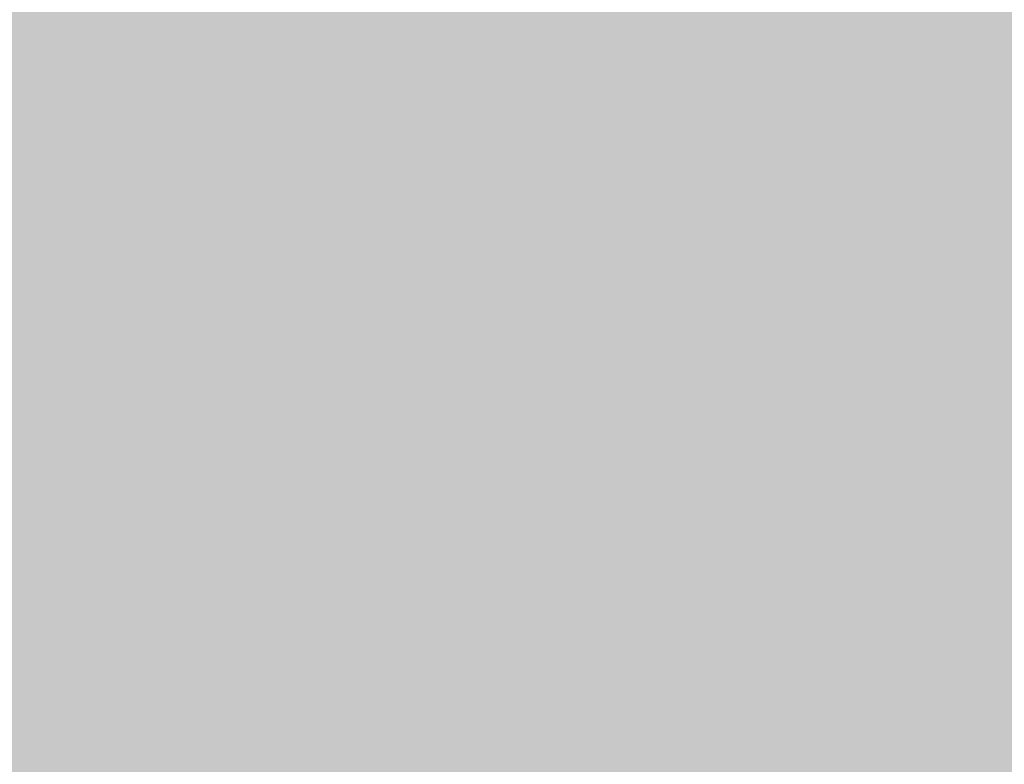
# Model space of a CAD drawing. Units: millimetres. Extents: x 0 to 2267, y 0 to 1823.
# Tile 45 of 256: x 1593.7801 to 1594.2193, y 1226.3857 to 1226.718. Entities that reach past the tile are written whole.
import ezdxf

# ---------------------------------------------------------------- set-up
doc = ezdxf.new("R2010")
doc.units = ezdxf.units.MM
doc.header["$MEASUREMENT"] = 0
doc.layers.add('M-HATC', color=252, linetype='Continuous', lineweight=18)

msp = doc.modelspace()

# ---------------------------------------------------------------- hatches: boundary and pattern name
at = {"layer": 'M-HATC'}
h = msp.add_hatch(color=256, dxfattribs=at)
h.dxf.hatch_style = 1
h.paths.add_polyline_path([(2055.77105, 1603.06204), (1381.08677, 1603.06204), (1381.08677, 1598.06204), (2055.77105, 1598.06204)])
h.paths.add_polyline_path([(2055.77105, 1598.06204), (1381.08677, 1598.06204), (1381.08677, 1593.06204), (2055.77105, 1593.06204)])
h.paths.add_polyline_path([(2051.30737, 1536.76088), (1385.55044, 1536.76088), (1385.55044, 1526.76088), (1387.55044, 1526.76088), (1388.53662, 1525.05276), (1385.33187, 1521.23348), (1385.33187, 1521.22256), (2050.25417, 1522.74913), (2048.32119, 1525.05276), (2049.30737, 1526.76088), (2051.30737, 1526.76088)])
edge = h.paths.add_edge_path()
edge.add_arc((1847.53451, 1379.14917), 135, 222.6030607, 222.8908505, ccw=False)
edge.add_line((1748.16629, 1287.76561), (1683.09212, 1287.76561))
edge.add_arc((1583.7239, 1379.14917), 135, 317.1091495, 317.3969393, ccw=False)
edge.add_arc((1678.9686, 1290.67067), 5, 222.89085, 317.10915, ccw=False)
edge.add_arc((1774.21331, 1379.14917), 135, 222.6030607, 222.8908505, ccw=False)
edge.add_line((1674.84509, 1287.76561), (1609.77092, 1287.76561))
edge.add_arc((1510.4027, 1379.14917), 135, 317.1091495, 317.3969393, ccw=False)
edge.add_arc((1605.6474, 1290.67067), 5, 222.89085, 317.10915, ccw=False)
edge.add_arc((1700.89211, 1379.14917), 135, 222.6030607, 222.8908505, ccw=False)
edge.add_line((1601.52388, 1287.76561), (1536.44972, 1287.76561))
edge.add_arc((1437.08149, 1379.14917), 135, 317.1091495, 317.3969393, ccw=False)
edge.add_arc((1532.3262, 1290.67067), 5, 222.89085, 317.10915, ccw=False)
edge.add_arc((1627.57091, 1379.14917), 135, 222.6030607, 222.8908505, ccw=False)
edge.add_line((1528.20268, 1287.76561), (1505.92891, 1287.76561))
edge.add_spline(control_points=[(1505.92891, 1287.76561), (1504.26224, 1287.76561), (1504.26224, 1282.76561), (1505.92891, 1282.76561)], knot_values=[0, 0, 0, 0, 5, 5, 5, 5], degree=3, periodic=0)
edge.add_line((1505.92891, 1282.76561), (1930.92891, 1282.76561))
edge.add_spline(control_points=[(1930.92891, 1282.76561), (1932.59557, 1282.76561), (1932.59557, 1287.76561), (1930.92891, 1287.76561)], knot_values=[0, 0, 0, 0, 5, 5, 5, 5], degree=3, periodic=0)
edge.add_line((1930.92891, 1287.76561), (1903.05573, 1287.76561))
edge.add_arc((1803.6875, 1379.14917), 135, 317.1091495, 317.3969393, ccw=False)
edge.add_arc((1898.93221, 1290.67067), 5, 222.89085, 317.10915, ccw=False)
edge.add_arc((1994.17691, 1379.14917), 135, 222.6030607, 222.8908505, ccw=False)
edge.add_line((1894.80869, 1287.76561), (1829.73452, 1287.76561))
edge.add_arc((1730.3663, 1379.14917), 135, 317.1091495, 317.3969393, ccw=False)
edge.add_arc((1825.61101, 1290.67067), 5, 222.89085, 317.10915, ccw=False)
edge.add_arc((1920.85571, 1379.14917), 135, 222.6030607, 222.8908505, ccw=False)
edge.add_line((1821.48749, 1287.76561), (1756.41332, 1287.76561))
edge.add_arc((1657.0451, 1379.14917), 135, 317.1091495, 317.3969393, ccw=False)
edge.add_arc((1752.28981, 1290.67067), 5, 222.89085, 317.10915, ccw=False)
edge = h.paths.add_edge_path()
edge.add_spline(control_points=[(1843.42891, 1227.24746), (1845.09557, 1227.24746), (1845.09557, 1232.24746), (1843.42891, 1232.24746)], knot_values=[0, 0, 0, 0, 5, 5, 5, 5], degree=3, periodic=0)
edge.add_line((1843.42891, 1232.24746), (1593.42891, 1232.24746))
edge.add_spline(control_points=[(1593.42891, 1232.24746), (1591.76224, 1232.24746), (1591.76224, 1227.24746), (1593.42891, 1227.24746)], knot_values=[0, 0, 0, 0, 5, 5, 5, 5], degree=3, periodic=0)
edge.add_line((1593.42891, 1227.24746), (1843.42891, 1227.24746))
h.paths.add_polyline_path([(1905.92891, 1127.41706), (1530.92891, 1127.41706, 0.414214), (1520.92891, 1117.41706), (1530.92891, 1117.41706), (1915.92891, 1117.41706, 0.414214)])
edge = h.paths.add_edge_path()
edge.add_arc((1397.08577, 1498.40775), 12.72993, 90.782146, 190.878706, ccw=False)
edge.add_line((1396.912, 1511.13649), (1428.00968, 1511.34875))
edge.add_line((1428.00968, 1511.34875), (1433.00968, 1511.34875))
edge.add_line((1433.00968, 1511.34875), (1434.439, 1511.34875))
edge.add_arc((1419.474, 1498.08041), 20, 41.560995, 74.082109)
edge.add_line((1424.95919, 1517.31353), (1399.93509, 1517.25608))
edge.add_spline(control_points=[(1399.93074, 1517.25607), (1399.88398, 1517.21312), (1399.8328, 1517.16893), (1399.77741, 1517.1236)], knot_values=[11.567499, 11.567499, 11.567499, 11.567499, 11.814249, 11.814249, 11.814249, 11.814249], degree=3, periodic=0)
edge.add_spline(control_points=[(1399.63279, 1517.00986), (1399.58305, 1516.97214), (1399.53072, 1516.93375), (1399.47591, 1516.89474)], knot_values=[11.167718, 11.167718, 11.167718, 11.167718, 11.365188, 11.365188, 11.365188, 11.365188], degree=3, periodic=0)
edge.add_spline(control_points=[(1399.33981, 1516.80007), (1399.15144, 1516.67185), (1398.93836, 1516.5377), (1398.70404, 1516.39942)], knot_values=[10.376405, 10.376405, 10.376405, 10.376405, 11.00994, 11.00994, 11.00994, 11.00994], degree=3, periodic=0)
edge.add_spline(control_points=[(1398.65716, 1516.37187), (1398.57885, 1516.32602), (1398.49825, 1516.27974), (1398.41549, 1516.23309)], knot_values=[10.125175, 10.125175, 10.125175, 10.125175, 10.334406, 10.334406, 10.334406, 10.334406], degree=3, periodic=0)
edge.add_spline(control_points=[(1398.26422, 1516.14874), (1398.19595, 1516.11107), (1398.12634, 1516.07319), (1398.05546, 1516.03513)], knot_values=[9.832246, 9.832246, 9.832246, 9.832246, 9.999658, 9.999658, 9.999658, 9.999658], degree=3, periodic=0)
edge.add_spline(control_points=[(1397.9987, 1516.00476), (1397.73115, 1515.86211), (1397.44602, 1515.71707), (1397.14664, 1515.57138)], knot_values=[9.161808, 9.161808, 9.161808, 9.161808, 9.787769, 9.787769, 9.787769, 9.787769], degree=3, periodic=0)
edge.add_spline(control_points=[(1397.14664, 1515.57138), (1396.84182, 1515.42305), (1396.52223, 1515.27404), (1396.1914, 1515.12621)], knot_values=[8.524455, 8.524455, 8.524455, 8.524455, 9.161808, 9.161808, 9.161808, 9.161808], degree=3, periodic=0)
edge.add_spline(control_points=[(1396.07771, 1515.07565), (1395.98538, 1515.03478), (1395.89222, 1514.99402), (1395.7983, 1514.9534)], knot_values=[8.275193, 8.275193, 8.275193, 8.275193, 8.451726, 8.451726, 8.451726, 8.451726], degree=3, periodic=0)
edge.add_spline(control_points=[(1395.60184, 1514.86912), (1395.49975, 1514.82568), (1395.39685, 1514.78244), (1395.29322, 1514.73944)], knot_values=[7.962917, 7.962917, 7.962917, 7.962917, 8.152764, 8.152764, 8.152764, 8.152764], degree=3, periodic=0)
edge.add_spline(control_points=[(1395.21158, 1514.70568), (1394.82779, 1514.5475), (1394.43452, 1514.39287), (1394.03645, 1514.24422)], knot_values=[7.21254, 7.21254, 7.21254, 7.21254, 7.913148, 7.913148, 7.913148, 7.913148], degree=3, periodic=0)
edge.add_spline(control_points=[(1394.03645, 1514.24422), (1393.70758, 1514.12142), (1393.37544, 1514.0027), (1393.04267, 1513.88945)], knot_values=[6.633733, 6.633733, 6.633733, 6.633733, 7.21254, 7.21254, 7.21254, 7.21254], degree=3, periodic=0)
edge.add_spline(control_points=[(1392.82142, 1513.81499), (1392.71978, 1513.78118), (1392.61815, 1513.74791), (1392.51658, 1513.71521)], knot_values=[6.328796, 6.328796, 6.328796, 6.328796, 6.505493, 6.505493, 6.505493, 6.505493], degree=3, periodic=0)
edge.add_spline(control_points=[(1392.51658, 1513.71521), (1392.31873, 1513.65151), (1392.12116, 1513.59001), (1391.92441, 1513.53098)], knot_values=[5.984605, 5.984605, 5.984605, 5.984605, 6.328796, 6.328796, 6.328796, 6.328796], degree=3, periodic=0)
edge.add_spline(control_points=[(1391.79155, 1513.49146), (1391.31215, 1513.35011), (1390.83842, 1513.22392), (1390.37844, 1513.11711)], knot_values=[5.066697, 5.066697, 5.066697, 5.066697, 5.907055, 5.907055, 5.907055, 5.907055], degree=3, periodic=0)
edge.add_spline(control_points=[(1390.37844, 1513.11711), (1390.17973, 1513.07097), (1389.98359, 1513.02845), (1389.79067, 1512.98988)], knot_values=[4.70367, 4.70367, 4.70367, 4.70367, 5.066695, 5.066695, 5.066695, 5.066695], degree=3, periodic=0)
edge.add_spline(control_points=[(1389.42203, 1512.92036), (1389.24588, 1512.88922), (1389.0729, 1512.86172), (1388.90364, 1512.83814)], knot_values=[4.130571, 4.130571, 4.130571, 4.130571, 4.469816, 4.469816, 4.469816, 4.469816], degree=3, periodic=0)
edge.add_spline(control_points=[(1388.90364, 1512.83814), (1388.59103, 1512.7946), (1388.29108, 1512.76444), (1388.00714, 1512.74941)], knot_values=[3.504031, 3.504031, 3.504031, 3.504031, 4.130571, 4.130571, 4.130571, 4.130571], degree=3, periodic=0)
edge.add_spline(control_points=[(1387.9356, 1512.74593), (1387.85378, 1512.74231), (1387.77334, 1512.73997), (1387.69435, 1512.73898)], knot_values=[3.268866, 3.268866, 3.268866, 3.268866, 3.451164, 3.451164, 3.451164, 3.451164], degree=3, periodic=0)
edge.add_spline(control_points=[(1387.33512, 1512.74426), (1387.20757, 1512.74991), (1387.08472, 1512.7597), (1386.96699, 1512.77385)], knot_values=[2.670686, 2.670686, 2.670686, 2.670686, 2.984, 2.984, 2.984, 2.984], degree=3, periodic=0)
edge.add_spline(control_points=[(1386.83274, 1512.79225), (1386.82093, 1512.79407), (1386.80917, 1512.79594), (1386.79747, 1512.79787)], knot_values=[2.516981, 2.516981, 2.516981, 2.516981, 2.549528, 2.549528, 2.549528, 2.549528], degree=3, periodic=0)
edge.add_spline(control_points=[(1386.45257, 1512.87348), (1386.42573, 1512.88105), (1386.39931, 1512.88895), (1386.3733, 1512.89719)], knot_values=[2.095869, 2.095869, 2.095869, 2.095869, 2.17941, 2.17941, 2.17941, 2.17941], degree=3, periodic=0)
edge.add_spline(control_points=[(1386.06911, 1513.01889), (1386.06338, 1513.02174), (1386.05768, 1513.02463), (1386.05201, 1513.02753)], knot_values=[1.72453, 1.72453, 1.72453, 1.72453, 1.745933, 1.745933, 1.745933, 1.745933], degree=3, periodic=0)
edge.add_arc((1399.474, 1498.08041), 20, 131.824322, 180)
edge.add_arc((1630.33362, 1505.54843), 250.97076, 181.7051759, 236.427975)
edge.add_arc((1605.33992, 1483.30441), 218.7822, 238.660829, 243.3496099)
edge.add_arc((1647.09105, 1510.35917), 262.89859, 183.1298361, 237.8534422, ccw=False)
h.paths.add_polyline_path([(1406.53685, 1391.96444, 0.149382), (1491.55061, 1296.44177, -0.129517)], flags=17)
edge = h.paths.add_edge_path()
edge.add_arc((2037.38381, 1498.08041), 20, 0, 48.265868)
edge.add_spline(control_points=[(2050.69731, 1513.00525), (2050.65121, 1512.98471), (2050.60338, 1512.96554), (2050.55388, 1512.94771)], knot_values=[1.835652, 1.835652, 1.835652, 1.835652, 2.000781, 2.000781, 2.000781, 2.000781], degree=3, periodic=0)
edge.add_spline(control_points=[(2050.46156, 1512.91661), (2050.479, 1512.9221), (2050.49625, 1512.92774), (2050.51332, 1512.93353)], knot_values=[2.045477, 2.045477, 2.045477, 2.045477, 2.101389, 2.101389, 2.101389, 2.101389], degree=3, periodic=0)
edge.add_spline(control_points=[(2050.12896, 1512.83416), (2050.19843, 1512.84734), (2050.26573, 1512.86233), (2050.33075, 1512.87919)], knot_values=[2.237629, 2.237629, 2.237629, 2.237629, 2.435841, 2.435841, 2.435841, 2.435841], degree=3, periodic=0)
edge.add_spline(control_points=[(2050.09463, 1512.82783), (2050.10613, 1512.82989), (2050.11757, 1512.832), (2050.12896, 1512.83416)], knot_values=[2.435841, 2.435841, 2.435841, 2.435841, 2.468321, 2.468321, 2.468321, 2.468321], degree=3, periodic=0)
edge.add_spline(control_points=[(2049.78433, 1512.78511), (2049.85521, 1512.79219), (2049.92435, 1512.80077), (2049.99166, 1512.81088)], knot_values=[2.563852, 2.563852, 2.563852, 2.563852, 2.748541, 2.748541, 2.748541, 2.748541], degree=3, periodic=0)
edge.add_spline(control_points=[(2049.4052, 1512.76169), (2049.5364, 1512.76526), (2049.66292, 1512.77299), (2049.78433, 1512.78511)], knot_values=[2.748541, 2.748541, 2.748541, 2.748541, 3.064882, 3.064882, 3.064882, 3.064882], degree=3, periodic=0)
edge.add_spline(control_points=[(2049.16976, 1512.75968), (2049.23364, 1512.7591), (2049.29654, 1512.7594), (2049.35844, 1512.7606)], knot_values=[3.102309, 3.102309, 3.102309, 3.102309, 3.2503, 3.2503, 3.2503, 3.2503], degree=3, periodic=0)
edge.add_spline(control_points=[(2048.85727, 1512.76911), (2048.96378, 1512.76378), (2049.068, 1512.76061), (2049.16976, 1512.75968)], knot_values=[3.2503, 3.2503, 3.2503, 3.2503, 3.486069, 3.486069, 3.486069, 3.486069], degree=3, periodic=0)
edge.add_spline(control_points=[(2048.69241, 1512.77892), (2048.3729, 1512.80093), (2048.0345, 1512.84106), (2047.68175, 1512.89697)], knot_values=[3.606429, 3.606429, 3.606429, 3.606429, 4.2989, 4.2989, 4.2989, 4.2989], degree=3, periodic=0)
edge.add_spline(control_points=[(2047.68175, 1512.89697), (2047.5458, 1512.91852), (2047.40772, 1512.94241), (2047.26776, 1512.96851)], knot_values=[4.2989, 4.2989, 4.2989, 4.2989, 4.565769, 4.565769, 4.565769, 4.565769], degree=3, periodic=0)
edge.add_spline(control_points=[(2047.26776, 1512.96851), (2047.14494, 1512.99141), (2047.02067, 1513.01601), (2046.89514, 1513.04223)], knot_values=[4.565769, 4.565769, 4.565769, 4.565769, 4.799971, 4.799971, 4.799971, 4.799971], degree=3, periodic=0)
edge.add_spline(control_points=[(2046.89514, 1513.04223), (2046.52865, 1513.11875), (2046.15135, 1513.20899), (2045.7676, 1513.31068)], knot_values=[4.799971, 4.799971, 4.799971, 4.799971, 5.483718, 5.483718, 5.483718, 5.483718], degree=3, periodic=0)
edge.add_spline(control_points=[(2045.7676, 1513.31068), (2045.3724, 1513.41539), (2044.97036, 1513.53225), (2044.56625, 1513.65876)], knot_values=[5.483718, 5.483718, 5.483718, 5.483718, 6.187866, 6.187866, 6.187866, 6.187866], degree=3, periodic=0)
edge.add_spline(control_points=[(2044.56625, 1513.65876), (2044.41491, 1513.70614), (2044.26329, 1513.75487), (2044.11163, 1513.80482)], knot_values=[6.187866, 6.187866, 6.187866, 6.187866, 6.451551, 6.451551, 6.451551, 6.451551], degree=3, periodic=0)
edge.add_spline(control_points=[(2044.11163, 1513.80482), (2043.99666, 1513.84269), (2043.88167, 1513.88126), (2043.76676, 1513.92048)], knot_values=[6.451551, 6.451551, 6.451551, 6.451551, 6.651434, 6.651434, 6.651434, 6.651434], degree=3, periodic=0)
edge.add_spline(control_points=[(2043.76676, 1513.92048), (2043.37157, 1514.05536), (2042.97738, 1514.19789), (2042.58863, 1514.34575)], knot_values=[6.651434, 6.651434, 6.651434, 6.651434, 7.338879, 7.338879, 7.338879, 7.338879], degree=3, periodic=0)
edge.add_spline(control_points=[(2042.58863, 1514.34575), (2042.16431, 1514.50715), (2041.74647, 1514.67491), (2041.34086, 1514.84603)], knot_values=[7.338879, 7.338879, 7.338879, 7.338879, 8.089209, 8.089209, 8.089209, 8.089209], degree=3, periodic=0)
edge.add_spline(control_points=[(2041.34086, 1514.84603), (2041.1028, 1514.94647), (2040.86896, 1515.04806), (2040.64049, 1515.1502)], knot_values=[8.089209, 8.089209, 8.089209, 8.089209, 8.529587, 8.529587, 8.529587, 8.529587], degree=3, periodic=0)
edge.add_spline(control_points=[(2040.50999, 1515.20887), (2040.08238, 1515.40218), (2039.67475, 1515.59705), (2039.29495, 1515.78939)], knot_values=[8.613818, 8.613818, 8.613818, 8.613818, 9.44571, 9.44571, 9.44571, 9.44571], degree=3, periodic=0)
edge.add_spline(control_points=[(2039.29495, 1515.78939), (2039.0618, 1515.90746), (2038.83914, 1516.02458), (2038.62878, 1516.1398)], knot_values=[9.44571, 9.44571, 9.44571, 9.44571, 9.956404, 9.956404, 9.956404, 9.956404], degree=3, periodic=0)
edge.add_spline(control_points=[(2038.62878, 1516.1398), (2038.51874, 1516.20007), (2038.41207, 1516.25982), (2038.30903, 1516.31891)], knot_values=[9.956404, 9.956404, 9.956404, 9.956404, 10.223542, 10.223542, 10.223542, 10.223542], degree=3, periodic=0)
edge.add_spline(control_points=[(2038.30903, 1516.31891), (2038.21377, 1516.37354), (2038.12161, 1516.42762), (2038.03275, 1516.48102)], knot_values=[10.223542, 10.223542, 10.223542, 10.223542, 10.47051, 10.47051, 10.47051, 10.47051], degree=3, periodic=0)
edge.add_spline(control_points=[(2038.03275, 1516.48102), (2037.78552, 1516.62961), (2037.56388, 1516.77304), (2037.37225, 1516.909)], knot_values=[10.47051, 10.47051, 10.47051, 10.47051, 11.15767, 11.15767, 11.15767, 11.15767], degree=3, periodic=0)
edge.add_spline(control_points=[(2037.37225, 1516.909), (2037.27893, 1516.9752), (2037.19274, 1517.03963), (2037.11417, 1517.10203)], knot_values=[11.15767, 11.15767, 11.15767, 11.15767, 11.49227, 11.49227, 11.49227, 11.49227], degree=3, periodic=0)
edge.add_spline(control_points=[(2036.85638, 1517.32585), (2036.91481, 1517.26923), (2036.98143, 1517.21027), (2037.05573, 1517.14922)], knot_values=[11.577341, 11.577341, 11.577341, 11.577341, 11.91035, 11.91035, 11.91035, 11.91035], degree=3, periodic=0)
edge.add_spline(control_points=[(2036.80739, 1517.37475), (2036.82301, 1517.35865), (2036.83935, 1517.34235), (2036.85638, 1517.32585)], knot_values=[11.91035, 11.91035, 11.91035, 11.91035, 12.007402, 12.007402, 12.007402, 12.007402], degree=3, periodic=0)
edge.add_spline(control_points=[(2036.70167, 1517.494), (2036.71042, 1517.48299), (2036.71958, 1517.47185), (2036.72913, 1517.4606)], knot_values=[12.184155, 12.184155, 12.184155, 12.184155, 12.255409, 12.255409, 12.255409, 12.255409], degree=3, periodic=0)
edge.add_spline(control_points=[(2036.6159, 1517.6205), (2036.61998, 1517.61304), (2036.6243, 1517.6055), (2036.62885, 1517.59789)], knot_values=[12.487913, 12.487913, 12.487913, 12.487913, 12.541035, 12.541035, 12.541035, 12.541035], degree=3, periodic=0)
edge.add_spline(control_points=[(2036.56349, 1517.78599), (2036.56372, 1517.77936), (2036.56423, 1517.77264), (2036.56502, 1517.76582)], knot_values=[12.911761, 12.911761, 12.911761, 12.911761, 12.968286, 12.968286, 12.968286, 12.968286], degree=3, periodic=0)
edge.add_spline(control_points=[(2036.61663, 1517.93042), (2036.61248, 1517.92586), (2036.60857, 1517.92121), (2036.60491, 1517.91648)], knot_values=[13.382527, 13.382527, 13.382527, 13.382527, 13.433791, 13.433791, 13.433791, 13.433791], degree=3, periodic=0)
edge.add_spline(control_points=[(2036.74902, 1518.01695), (2036.73613, 1518.0116), (2036.72393, 1518.00601), (2036.71242, 1518.00018)], knot_values=[13.726299, 13.726299, 13.726299, 13.726299, 13.809928, 13.809928, 13.809928, 13.809928], degree=3, periodic=0)
edge.add_spline(control_points=[(2036.86043, 1518.05285), (2036.83863, 1518.04743), (2036.81809, 1518.04156), (2036.79879, 1518.03526)], knot_values=[13.910887, 13.910887, 13.910887, 13.910887, 14.02153, 14.02153, 14.02153, 14.02153], degree=3, periodic=0)
edge.add_line((2036.96387, 1518.08041), (2032.38381, 1518.08041))
edge.add_line((2032.38381, 1518.08041), (2027.38381, 1518.08041))
edge.add_line((2027.38381, 1518.08041), (2022.38381, 1518.08041))
edge.add_line((2022.38381, 1518.08041), (2017.38381, 1518.08041))
edge.add_arc((2017.38381, 1498.08041), 20, 90, 138.439005)
edge.add_line((2002.41881, 1511.34875), (2003.84813, 1511.34875))
edge.add_line((2003.84813, 1511.34875), (2008.84813, 1511.34875))
edge.add_line((2008.84813, 1511.34875), (2039.77204, 1511.13768))
edge.add_arc((2039.77204, 1498.40775), 12.72993, -10.878706, 90, ccw=False)
edge.add_arc((1789.76676, 1510.35917), 262.89859, 302.1465578, 356.8701639, ccw=False)
edge.add_arc((1831.51789, 1483.30441), 218.7822, 296.6503901, 301.339171)
edge.add_arc((1806.52419, 1505.54843), 250.97076, 303.572025, 358.2948241)
h.paths.add_polyline_path([(2030.32096, 1391.96444, -0.129517), (1945.3072, 1296.44177, 0.149382)], flags=17)
edge = h.paths.add_edge_path()
edge.add_spline(control_points=[(2037.2464, 1518.08209), (2037.28977, 1518.08098), (2037.33555, 1518.08041), (2037.3838, 1518.08041)], knot_values=[0.000012, 0.000012, 0.000012, 0.000012, 0.144754, 0.144754, 0.144754, 0.144754], degree=3, periodic=0)
edge.add_line((2037.33571, 1518.08041), (2037.00963, 1518.08041))
edge.add_spline(control_points=[(2037.00963, 1518.08041), (2036.98217, 1518.07678), (2036.95605, 1518.07266), (2036.93124, 1518.06808)], knot_values=[14.13465, 14.13465, 14.13465, 14.13465, 14.247197, 14.247197, 14.247197, 14.247197], degree=3, periodic=0)
edge.add_spline(control_points=[(2036.93124, 1518.06808), (2036.92764, 1518.06741), (2036.92407, 1518.06674), (2036.92053, 1518.06605)], knot_values=[14.118315, 14.118315, 14.118315, 14.118315, 14.13465, 14.13465, 14.13465, 14.13465], degree=3, periodic=0)
edge.add_spline(control_points=[(2036.92053, 1518.06605), (2036.9118, 1518.06436), (2036.90323, 1518.06262), (2036.89484, 1518.06081)], knot_values=[14.078086, 14.078086, 14.078086, 14.078086, 14.118315, 14.118315, 14.118315, 14.118315], degree=3, periodic=0)
edge.add_spline(control_points=[(2036.89484, 1518.06081), (2036.88304, 1518.05827), (2036.87157, 1518.05562), (2036.86043, 1518.05285)], knot_values=[14.02153, 14.02153, 14.02153, 14.02153, 14.078086, 14.078086, 14.078086, 14.078086], degree=3, periodic=0)
edge.add_spline(control_points=[(2036.86043, 1518.05285), (2036.83863, 1518.04743), (2036.81809, 1518.04156), (2036.79879, 1518.03526)], knot_values=[13.910887, 13.910887, 13.910887, 13.910887, 14.02153, 14.02153, 14.02153, 14.02153], degree=3, periodic=0)
edge.add_spline(control_points=[(2036.79879, 1518.03526), (2036.79809, 1518.03504), (2036.7974, 1518.03481), (2036.79671, 1518.03458)], knot_values=[13.906906, 13.906906, 13.906906, 13.906906, 13.910887, 13.910887, 13.910887, 13.910887], degree=3, periodic=0)
edge.add_spline(control_points=[(2036.79671, 1518.03458), (2036.78819, 1518.03178), (2036.77991, 1518.02888), (2036.77187, 1518.02591)], knot_values=[13.857826, 13.857826, 13.857826, 13.857826, 13.906906, 13.906906, 13.906906, 13.906906], degree=3, periodic=0)
edge.add_spline(control_points=[(2036.77187, 1518.02591), (2036.76402, 1518.023), (2036.75641, 1518.02002), (2036.74902, 1518.01695)], knot_values=[13.809928, 13.809928, 13.809928, 13.809928, 13.857826, 13.857826, 13.857826, 13.857826], degree=3, periodic=0)
edge.add_spline(control_points=[(2036.74902, 1518.01695), (2036.73613, 1518.0116), (2036.72393, 1518.00601), (2036.71242, 1518.00018)], knot_values=[13.726299, 13.726299, 13.726299, 13.726299, 13.809928, 13.809928, 13.809928, 13.809928], degree=3, periodic=0)
edge.add_spline(control_points=[(2036.71242, 1518.00018), (2036.71211, 1518.00002), (2036.71179, 1517.99986), (2036.71147, 1517.99969)], knot_values=[13.723993, 13.723993, 13.723993, 13.723993, 13.726299, 13.726299, 13.726299, 13.726299], degree=3, periodic=0)
edge.add_spline(control_points=[(2036.71147, 1517.99969), (2036.70634, 1517.99708), (2036.70134, 1517.99441), (2036.69648, 1517.9917)], knot_values=[13.686536, 13.686536, 13.686536, 13.686536, 13.723993, 13.723993, 13.723993, 13.723993], degree=3, periodic=0)
edge.add_spline(control_points=[(2036.69648, 1517.9917), (2036.6919, 1517.98914), (2036.68744, 1517.98654), (2036.6831, 1517.9839)], knot_values=[13.651251, 13.651251, 13.651251, 13.651251, 13.686536, 13.686536, 13.686536, 13.686536], degree=3, periodic=0)
edge.add_spline(control_points=[(2036.6831, 1517.9839), (2036.67641, 1517.97983), (2036.67001, 1517.97566), (2036.6639, 1517.97139)], knot_values=[13.596804, 13.596804, 13.596804, 13.596804, 13.651251, 13.651251, 13.651251, 13.651251], degree=3, periodic=0)
edge.add_spline(control_points=[(2036.6639, 1517.97139), (2036.66358, 1517.97117), (2036.66326, 1517.97094), (2036.66294, 1517.97072)], knot_values=[13.593956, 13.593956, 13.593956, 13.593956, 13.596804, 13.596804, 13.596804, 13.596804], degree=3, periodic=0)
edge.add_spline(control_points=[(2036.66294, 1517.97072), (2036.6603, 1517.96886), (2036.65771, 1517.96698), (2036.65518, 1517.96509)], knot_values=[13.570322, 13.570322, 13.570322, 13.570322, 13.593956, 13.593956, 13.593956, 13.593956], degree=3, periodic=0)
edge.add_spline(control_points=[(2036.65518, 1517.96509), (2036.65251, 1517.9631), (2036.64991, 1517.96108), (2036.64737, 1517.95905)], knot_values=[13.545477, 13.545477, 13.545477, 13.545477, 13.570322, 13.570322, 13.570322, 13.570322], degree=3, periodic=0)
edge.add_spline(control_points=[(2036.64737, 1517.95905), (2036.64721, 1517.95892), (2036.64705, 1517.9588), (2036.64689, 1517.95867)], knot_values=[13.543931, 13.543931, 13.543931, 13.543931, 13.545477, 13.545477, 13.545477, 13.545477], degree=3, periodic=0)
edge.add_spline(control_points=[(2036.64689, 1517.95867), (2036.64121, 1517.95411), (2036.63582, 1517.94945), (2036.63073, 1517.94468)], knot_values=[13.488237, 13.488237, 13.488237, 13.488237, 13.543931, 13.543931, 13.543931, 13.543931], degree=3, periodic=0)
edge.add_spline(control_points=[(2036.63073, 1517.94468), (2036.62817, 1517.94229), (2036.62569, 1517.93988), (2036.62329, 1517.93744)], knot_values=[13.460307, 13.460307, 13.460307, 13.460307, 13.488237, 13.488237, 13.488237, 13.488237], degree=3, periodic=0)
edge.add_spline(control_points=[(2036.62329, 1517.93744), (2036.62151, 1517.93564), (2036.61978, 1517.93383), (2036.61809, 1517.932)], knot_values=[13.439712, 13.439712, 13.439712, 13.439712, 13.460307, 13.460307, 13.460307, 13.460307], degree=3, periodic=0)
edge.add_spline(control_points=[(2036.61809, 1517.932), (2036.6176, 1517.93147), (2036.61711, 1517.93095), (2036.61663, 1517.93042)], knot_values=[13.433791, 13.433791, 13.433791, 13.433791, 13.439712, 13.439712, 13.439712, 13.439712], degree=3, periodic=0)
edge.add_spline(control_points=[(2036.61663, 1517.93042), (2036.61248, 1517.92586), (2036.60857, 1517.92121), (2036.60491, 1517.91648)], knot_values=[13.382527, 13.382527, 13.382527, 13.382527, 13.433791, 13.433791, 13.433791, 13.433791], degree=3, periodic=0)
edge.add_spline(control_points=[(2036.60491, 1517.91648), (2036.60258, 1517.91347), (2036.60036, 1517.91044), (2036.59824, 1517.90737)], knot_values=[13.350017, 13.350017, 13.350017, 13.350017, 13.382527, 13.382527, 13.382527, 13.382527], degree=3, periodic=0)
edge.add_spline(control_points=[(2036.59824, 1517.90737), (2036.59718, 1517.90585), (2036.59616, 1517.90433), (2036.59515, 1517.90279)], knot_values=[13.333922, 13.333922, 13.333922, 13.333922, 13.350017, 13.350017, 13.350017, 13.350017], degree=3, periodic=0)
edge.add_spline(control_points=[(2036.59515, 1517.90279), (2036.59452, 1517.90183), (2036.5939, 1517.90086), (2036.59329, 1517.89989)], knot_values=[13.323828, 13.323828, 13.323828, 13.323828, 13.333922, 13.333922, 13.333922, 13.333922], degree=3, periodic=0)
edge.add_spline(control_points=[(2036.59329, 1517.89989), (2036.59049, 1517.89545), (2036.5879, 1517.89094), (2036.5855, 1517.88637)], knot_values=[13.277545, 13.277545, 13.277545, 13.277545, 13.323828, 13.323828, 13.323828, 13.323828], degree=3, periodic=0)
edge.add_spline(control_points=[(2036.5855, 1517.88637), (2036.58355, 1517.88267), (2036.58174, 1517.87892), (2036.58006, 1517.87513)], knot_values=[13.240119, 13.240119, 13.240119, 13.240119, 13.277545, 13.277545, 13.277545, 13.277545], degree=3, periodic=0)
edge.add_spline(control_points=[(2036.58006, 1517.87513), (2036.57952, 1517.87393), (2036.579, 1517.87272), (2036.57849, 1517.87151)], knot_values=[13.228211, 13.228211, 13.228211, 13.228211, 13.240119, 13.240119, 13.240119, 13.240119], degree=3, periodic=0)
edge.add_spline(control_points=[(2036.57849, 1517.87151), (2036.57796, 1517.87023), (2036.57744, 1517.86896), (2036.57693, 1517.86767)], knot_values=[13.215717, 13.215717, 13.215717, 13.215717, 13.228211, 13.228211, 13.228211, 13.228211], degree=3, periodic=0)
edge.add_spline(control_points=[(2036.57693, 1517.86767), (2036.57548, 1517.86399), (2036.57414, 1517.86027), (2036.57293, 1517.85651)], knot_values=[13.179847, 13.179847, 13.179847, 13.179847, 13.215717, 13.215717, 13.215717, 13.215717], degree=3, periodic=0)
edge.add_spline(control_points=[(2036.57293, 1517.85651), (2036.5713, 1517.8515), (2036.56989, 1517.84641), (2036.56868, 1517.84126)], knot_values=[13.132017, 13.132017, 13.132017, 13.132017, 13.179847, 13.179847, 13.179847, 13.179847], degree=3, periodic=0)
edge.add_spline(control_points=[(2036.56868, 1517.84126), (2036.56844, 1517.84023), (2036.56821, 1517.8392), (2036.56798, 1517.83817)], knot_values=[13.122482, 13.122482, 13.122482, 13.122482, 13.132017, 13.132017, 13.132017, 13.132017], degree=3, periodic=0)
edge.add_spline(control_points=[(2036.56798, 1517.83817), (2036.56758, 1517.83634), (2036.56721, 1517.8345), (2036.56687, 1517.83266)], knot_values=[13.105592, 13.105592, 13.105592, 13.105592, 13.122482, 13.122482, 13.122482, 13.122482], degree=3, periodic=0)
edge.add_spline(control_points=[(2036.56687, 1517.83266), (2036.56622, 1517.82921), (2036.56567, 1517.82574), (2036.5652, 1517.82223)], knot_values=[13.074063, 13.074063, 13.074063, 13.074063, 13.105592, 13.105592, 13.105592, 13.105592], degree=3, periodic=0)
edge.add_spline(control_points=[(2036.5652, 1517.82223), (2036.5652, 1517.82223), (2036.5652, 1517.82223), (2036.5652, 1517.82223)], knot_values=[13.074043, 13.074043, 13.074043, 13.074043, 13.074063, 13.074063, 13.074063, 13.074063], degree=3, periodic=0)
edge.add_spline(control_points=[(2036.5652, 1517.82223), (2036.56443, 1517.81643), (2036.5639, 1517.81055), (2036.56361, 1517.8046)], knot_values=[13.021884, 13.021884, 13.021884, 13.021884, 13.074043, 13.074043, 13.074043, 13.074043], degree=3, periodic=0)
edge.add_spline(control_points=[(2036.56361, 1517.8046), (2036.56358, 1517.80401), (2036.56356, 1517.80342), (2036.56353, 1517.80283)], knot_values=[13.01674, 13.01674, 13.01674, 13.01674, 13.021884, 13.021884, 13.021884, 13.021884], degree=3, periodic=0)
edge.add_spline(control_points=[(2036.56353, 1517.80283), (2036.56344, 1517.80051), (2036.56338, 1517.79817), (2036.56336, 1517.79582)], knot_values=[12.996438, 12.996438, 12.996438, 12.996438, 13.01674, 13.01674, 13.01674, 13.01674], degree=3, periodic=0)
edge.add_spline(control_points=[(2036.56336, 1517.79582), (2036.56334, 1517.79257), (2036.56338, 1517.78929), (2036.56349, 1517.78599)], knot_values=[12.968286, 12.968286, 12.968286, 12.968286, 12.996438, 12.996438, 12.996438, 12.996438], degree=3, periodic=0)
edge.add_spline(control_points=[(2036.56349, 1517.78599), (2036.56372, 1517.77936), (2036.56423, 1517.77264), (2036.56502, 1517.76582)], knot_values=[12.911761, 12.911761, 12.911761, 12.911761, 12.968286, 12.968286, 12.968286, 12.968286], degree=3, periodic=0)
edge.add_spline(control_points=[(2036.56502, 1517.76582), (2036.56503, 1517.76573), (2036.56504, 1517.76564), (2036.56505, 1517.76555)], knot_values=[12.911017, 12.911017, 12.911017, 12.911017, 12.911761, 12.911761, 12.911761, 12.911761], degree=3, periodic=0)
edge.add_spline(control_points=[(2036.56505, 1517.76555), (2036.56541, 1517.76245), (2036.56583, 1517.75933), (2036.56631, 1517.75619)], knot_values=[12.88528, 12.88528, 12.88528, 12.88528, 12.911017, 12.911017, 12.911017, 12.911017], degree=3, periodic=0)
edge.add_spline(control_points=[(2036.56631, 1517.75619), (2036.56673, 1517.75341), (2036.5672, 1517.75062), (2036.56771, 1517.74782)], knot_values=[12.862519, 12.862519, 12.862519, 12.862519, 12.88528, 12.88528, 12.88528, 12.88528], degree=3, periodic=0)
edge.add_spline(control_points=[(2036.56771, 1517.74782), (2036.56779, 1517.74737), (2036.56788, 1517.74692), (2036.56796, 1517.74647)], knot_values=[12.858885, 12.858885, 12.858885, 12.858885, 12.862519, 12.862519, 12.862519, 12.862519], degree=3, periodic=0)
edge.add_spline(control_points=[(2036.56796, 1517.74647), (2036.5692, 1517.73986), (2036.57069, 1517.73316), (2036.57243, 1517.72638)], knot_values=[12.8053, 12.8053, 12.8053, 12.8053, 12.858885, 12.858885, 12.858885, 12.858885], degree=3, periodic=0)
edge.add_spline(control_points=[(2036.57243, 1517.72638), (2036.5734, 1517.72257), (2036.57446, 1517.71874), (2036.57559, 1517.71488)], knot_values=[12.775176, 12.775176, 12.775176, 12.775176, 12.8053, 12.8053, 12.8053, 12.8053], degree=3, periodic=0)
edge.add_spline(control_points=[(2036.57559, 1517.71488), (2036.57628, 1517.71252), (2036.577, 1517.71015), (2036.57775, 1517.70778)], knot_values=[12.756759, 12.756759, 12.756759, 12.756759, 12.775176, 12.775176, 12.775176, 12.775176], degree=3, periodic=0)
edge.add_spline(control_points=[(2036.57775, 1517.70778), (2036.57808, 1517.70674), (2036.57841, 1517.7057), (2036.57875, 1517.70466)], knot_values=[12.748742, 12.748742, 12.748742, 12.748742, 12.756759, 12.756759, 12.756759, 12.756759], degree=3, periodic=0)
edge.add_spline(control_points=[(2036.57875, 1517.70466), (2036.58082, 1517.6983), (2036.58309, 1517.69187), (2036.58557, 1517.68537)], knot_values=[12.69959, 12.69959, 12.69959, 12.69959, 12.748742, 12.748742, 12.748742, 12.748742], degree=3, periodic=0)
edge.add_spline(control_points=[(2036.58557, 1517.68537), (2036.58762, 1517.68001), (2036.5898, 1517.6746), (2036.59213, 1517.66916)], knot_values=[12.659038, 12.659038, 12.659038, 12.659038, 12.69959, 12.69959, 12.69959, 12.69959], degree=3, periodic=0)
edge.add_spline(control_points=[(2036.59213, 1517.66916), (2036.59397, 1517.66482), (2036.59591, 1517.66047), (2036.59793, 1517.65608)], knot_values=[12.626806, 12.626806, 12.626806, 12.626806, 12.659038, 12.659038, 12.659038, 12.659038], degree=3, periodic=0)
edge.add_spline(control_points=[(2036.59793, 1517.65608), (2036.59839, 1517.65507), (2036.59886, 1517.65406), (2036.59934, 1517.65305)], knot_values=[12.619394, 12.619394, 12.619394, 12.619394, 12.626806, 12.626806, 12.626806, 12.626806], degree=3, periodic=0)
edge.add_spline(control_points=[(2036.59934, 1517.65305), (2036.60435, 1517.64236), (2036.60987, 1517.63151), (2036.61589, 1517.6205)], knot_values=[12.541039, 12.541039, 12.541039, 12.541039, 12.619394, 12.619394, 12.619394, 12.619394], degree=3, periodic=0)
edge.add_spline(control_points=[(2036.61589, 1517.6205), (2036.61589, 1517.6205), (2036.6159, 1517.6205), (2036.6159, 1517.6205)], knot_values=[12.541035, 12.541035, 12.541035, 12.541035, 12.541039, 12.541039, 12.541039, 12.541039], degree=3, periodic=0)
edge.add_spline(control_points=[(2036.6159, 1517.6205), (2036.61998, 1517.61304), (2036.6243, 1517.6055), (2036.62885, 1517.59789)], knot_values=[12.487913, 12.487913, 12.487913, 12.487913, 12.541035, 12.541035, 12.541035, 12.541035], degree=3, periodic=0)
edge.add_spline(control_points=[(2036.62885, 1517.59789), (2036.63261, 1517.5916), (2036.63653, 1517.58526), (2036.64061, 1517.57888)], knot_values=[12.443982, 12.443982, 12.443982, 12.443982, 12.487913, 12.487913, 12.487913, 12.487913], degree=3, periodic=0)
edge.add_spline(control_points=[(2036.64061, 1517.57888), (2036.64144, 1517.57757), (2036.64228, 1517.57626), (2036.64313, 1517.57495)], knot_values=[12.434996, 12.434996, 12.434996, 12.434996, 12.443982, 12.443982, 12.443982, 12.443982], degree=3, periodic=0)
edge.add_spline(control_points=[(2036.64313, 1517.57495), (2036.65306, 1517.55958), (2036.66389, 1517.54394), (2036.6756, 1517.52803)], knot_values=[12.329647, 12.329647, 12.329647, 12.329647, 12.434996, 12.434996, 12.434996, 12.434996], degree=3, periodic=0)
edge.add_spline(control_points=[(2036.6756, 1517.52803), (2036.68385, 1517.51682), (2036.69254, 1517.50548), (2036.70167, 1517.494)], knot_values=[12.255409, 12.255409, 12.255409, 12.255409, 12.329647, 12.329647, 12.329647, 12.329647], degree=3, periodic=0)
edge.add_spline(control_points=[(2036.70167, 1517.494), (2036.71042, 1517.48299), (2036.71958, 1517.47185), (2036.72913, 1517.4606)], knot_values=[12.184155, 12.184155, 12.184155, 12.184155, 12.255409, 12.255409, 12.255409, 12.255409], degree=3, periodic=0)
edge.add_spline(control_points=[(2036.72913, 1517.4606), (2036.74363, 1517.44352), (2036.75904, 1517.42617), (2036.77534, 1517.40855)], knot_values=[12.075961, 12.075961, 12.075961, 12.075961, 12.184155, 12.184155, 12.184155, 12.184155], degree=3, periodic=0)
edge.add_spline(control_points=[(2036.77534, 1517.40855), (2036.77631, 1517.4075), (2036.77729, 1517.40645), (2036.77827, 1517.40539)], knot_values=[12.069502, 12.069502, 12.069502, 12.069502, 12.075961, 12.075961, 12.075961, 12.075961], degree=3, periodic=0)
edge.add_spline(control_points=[(2036.77827, 1517.40539), (2036.78768, 1517.39526), (2036.79739, 1517.38505), (2036.80739, 1517.37475)], knot_values=[12.007402, 12.007402, 12.007402, 12.007402, 12.069502, 12.069502, 12.069502, 12.069502], degree=3, periodic=0)
edge.add_spline(control_points=[(2036.80739, 1517.37475), (2036.82301, 1517.35865), (2036.83935, 1517.34235), (2036.85638, 1517.32585)], knot_values=[11.91035, 11.91035, 11.91035, 11.91035, 12.007402, 12.007402, 12.007402, 12.007402], degree=3, periodic=0)
edge.add_spline(control_points=[(2036.85638, 1517.32585), (2036.91481, 1517.26923), (2036.98143, 1517.21027), (2037.05573, 1517.14922)], knot_values=[11.577341, 11.577341, 11.577341, 11.577341, 11.91035, 11.91035, 11.91035, 11.91035], degree=3, periodic=0)
edge.add_spline(control_points=[(2037.05573, 1517.14922), (2037.07471, 1517.13362), (2037.0942, 1517.11789), (2037.11417, 1517.10203)], knot_values=[11.49227, 11.49227, 11.49227, 11.49227, 11.577341, 11.577341, 11.577341, 11.577341], degree=3, periodic=0)
edge.add_spline(control_points=[(2037.11417, 1517.10203), (2037.19274, 1517.03963), (2037.27893, 1516.9752), (2037.37225, 1516.909)], knot_values=[11.15767, 11.15767, 11.15767, 11.15767, 11.49227, 11.49227, 11.49227, 11.49227], degree=3, periodic=0)
edge.add_spline(control_points=[(2037.37225, 1516.909), (2037.56388, 1516.77304), (2037.78552, 1516.62961), (2038.03275, 1516.48102)], knot_values=[10.47051, 10.47051, 10.47051, 10.47051, 11.15767, 11.15767, 11.15767, 11.15767], degree=3, periodic=0)
edge.add_spline(control_points=[(2038.03275, 1516.48102), (2038.12161, 1516.42762), (2038.21377, 1516.37354), (2038.30903, 1516.31891)], knot_values=[10.223542, 10.223542, 10.223542, 10.223542, 10.47051, 10.47051, 10.47051, 10.47051], degree=3, periodic=0)
edge.add_spline(control_points=[(2038.30903, 1516.31891), (2038.41207, 1516.25982), (2038.51874, 1516.20007), (2038.62878, 1516.1398)], knot_values=[9.956404, 9.956404, 9.956404, 9.956404, 10.223542, 10.223542, 10.223542, 10.223542], degree=3, periodic=0)
edge.add_spline(control_points=[(2038.62878, 1516.1398), (2038.83914, 1516.02458), (2039.0618, 1515.90746), (2039.29495, 1515.78939)], knot_values=[9.44571, 9.44571, 9.44571, 9.44571, 9.956404, 9.956404, 9.956404, 9.956404], degree=3, periodic=0)
edge.add_spline(control_points=[(2039.29495, 1515.78939), (2039.67475, 1515.59705), (2040.08238, 1515.40218), (2040.50999, 1515.20887)], knot_values=[8.613818, 8.613818, 8.613818, 8.613818, 9.44571, 9.44571, 9.44571, 9.44571], degree=3, periodic=0)
edge.add_spline(control_points=[(2040.50999, 1515.20887), (2040.55329, 1515.1893), (2040.59679, 1515.16974), (2040.64049, 1515.1502)], knot_values=[8.529587, 8.529587, 8.529587, 8.529587, 8.613818, 8.613818, 8.613818, 8.613818], degree=3, periodic=0)
edge.add_spline(control_points=[(2040.64049, 1515.1502), (2040.86896, 1515.04806), (2041.1028, 1514.94647), (2041.34086, 1514.84603)], knot_values=[8.089209, 8.089209, 8.089209, 8.089209, 8.529587, 8.529587, 8.529587, 8.529587], degree=3, periodic=0)
edge.add_spline(control_points=[(2041.34086, 1514.84603), (2041.74647, 1514.67491), (2042.16431, 1514.50715), (2042.58863, 1514.34575)], knot_values=[7.338879, 7.338879, 7.338879, 7.338879, 8.089209, 8.089209, 8.089209, 8.089209], degree=3, periodic=0)
edge.add_spline(control_points=[(2042.58863, 1514.34575), (2042.97738, 1514.19789), (2043.37157, 1514.05536), (2043.76676, 1513.92048)], knot_values=[6.651434, 6.651434, 6.651434, 6.651434, 7.338879, 7.338879, 7.338879, 7.338879], degree=3, periodic=0)
edge.add_spline(control_points=[(2043.76676, 1513.92048), (2043.88167, 1513.88126), (2043.99666, 1513.84269), (2044.11163, 1513.80482)], knot_values=[6.451551, 6.451551, 6.451551, 6.451551, 6.651434, 6.651434, 6.651434, 6.651434], degree=3, periodic=0)
edge.add_spline(control_points=[(2044.11163, 1513.80482), (2044.26329, 1513.75487), (2044.41491, 1513.70614), (2044.56625, 1513.65876)], knot_values=[6.187866, 6.187866, 6.187866, 6.187866, 6.451551, 6.451551, 6.451551, 6.451551], degree=3, periodic=0)
edge.add_spline(control_points=[(2044.56625, 1513.65876), (2044.97036, 1513.53225), (2045.3724, 1513.41539), (2045.7676, 1513.31068)], knot_values=[5.483718, 5.483718, 5.483718, 5.483718, 6.187866, 6.187866, 6.187866, 6.187866], degree=3, periodic=0)
edge.add_spline(control_points=[(2045.7676, 1513.31068), (2046.15135, 1513.20899), (2046.52865, 1513.11875), (2046.89514, 1513.04223)], knot_values=[4.799971, 4.799971, 4.799971, 4.799971, 5.483718, 5.483718, 5.483718, 5.483718], degree=3, periodic=0)
edge.add_spline(control_points=[(2046.89514, 1513.04223), (2047.02067, 1513.01601), (2047.14494, 1512.99141), (2047.26776, 1512.96851)], knot_values=[4.565769, 4.565769, 4.565769, 4.565769, 4.799971, 4.799971, 4.799971, 4.799971], degree=3, periodic=0)
edge.add_spline(control_points=[(2047.26776, 1512.96851), (2047.40772, 1512.94241), (2047.5458, 1512.91852), (2047.68175, 1512.89697)], knot_values=[4.2989, 4.2989, 4.2989, 4.2989, 4.565769, 4.565769, 4.565769, 4.565769], degree=3, periodic=0)
edge.add_spline(control_points=[(2047.68175, 1512.89697), (2048.0345, 1512.84106), (2048.3729, 1512.80093), (2048.69241, 1512.77892)], knot_values=[3.606429, 3.606429, 3.606429, 3.606429, 4.2989, 4.2989, 4.2989, 4.2989], degree=3, periodic=0)
edge.add_spline(control_points=[(2048.69241, 1512.77892), (2048.74794, 1512.7751), (2048.8029, 1512.77182), (2048.85727, 1512.76911)], knot_values=[3.486069, 3.486069, 3.486069, 3.486069, 3.606429, 3.606429, 3.606429, 3.606429], degree=3, periodic=0)
edge.add_spline(control_points=[(2048.85727, 1512.76911), (2048.96378, 1512.76378), (2049.068, 1512.76061), (2049.16976, 1512.75968)], knot_values=[3.2503, 3.2503, 3.2503, 3.2503, 3.486069, 3.486069, 3.486069, 3.486069], degree=3, periodic=0)
edge.add_spline(control_points=[(2049.16976, 1512.75968), (2049.23364, 1512.7591), (2049.29654, 1512.7594), (2049.35844, 1512.7606)], knot_values=[3.102309, 3.102309, 3.102309, 3.102309, 3.2503, 3.2503, 3.2503, 3.2503], degree=3, periodic=0)
edge.add_spline(control_points=[(2049.35844, 1512.7606), (2049.37409, 1512.76091), (2049.38968, 1512.76127), (2049.4052, 1512.76169)], knot_values=[3.064882, 3.064882, 3.064882, 3.064882, 3.102309, 3.102309, 3.102309, 3.102309], degree=3, periodic=0)
edge.add_spline(control_points=[(2049.4052, 1512.76169), (2049.5364, 1512.76526), (2049.66292, 1512.77299), (2049.78433, 1512.78511)], knot_values=[2.748541, 2.748541, 2.748541, 2.748541, 3.064882, 3.064882, 3.064882, 3.064882], degree=3, periodic=0)
edge.add_spline(control_points=[(2049.78433, 1512.78511), (2049.85521, 1512.79219), (2049.92435, 1512.80077), (2049.99166, 1512.81088)], knot_values=[2.563852, 2.563852, 2.563852, 2.563852, 2.748541, 2.748541, 2.748541, 2.748541], degree=3, periodic=0)
edge.add_spline(control_points=[(2049.99166, 1512.81088), (2050.02648, 1512.81612), (2050.0608, 1512.82177), (2050.09463, 1512.82783)], knot_values=[2.468321, 2.468321, 2.468321, 2.468321, 2.563852, 2.563852, 2.563852, 2.563852], degree=3, periodic=0)
edge.add_spline(control_points=[(2050.09463, 1512.82783), (2050.10613, 1512.82989), (2050.11757, 1512.832), (2050.12896, 1512.83416)], knot_values=[2.435841, 2.435841, 2.435841, 2.435841, 2.468321, 2.468321, 2.468321, 2.468321], degree=3, periodic=0)
edge.add_spline(control_points=[(2050.12896, 1512.83416), (2050.19843, 1512.84734), (2050.26573, 1512.86233), (2050.33075, 1512.87919)], knot_values=[2.237629, 2.237629, 2.237629, 2.237629, 2.435841, 2.435841, 2.435841, 2.435841], degree=3, periodic=0)
edge.add_spline(control_points=[(2050.33075, 1512.87919), (2050.37544, 1512.89077), (2050.41906, 1512.90324), (2050.46156, 1512.91661)], knot_values=[2.101389, 2.101389, 2.101389, 2.101389, 2.237629, 2.237629, 2.237629, 2.237629], degree=3, periodic=0)
edge.add_spline(control_points=[(2050.46156, 1512.91661), (2050.479, 1512.9221), (2050.49625, 1512.92774), (2050.51332, 1512.93353)], knot_values=[2.045477, 2.045477, 2.045477, 2.045477, 2.101389, 2.101389, 2.101389, 2.101389], degree=3, periodic=0)
edge.add_spline(control_points=[(2050.51332, 1512.93353), (2050.52696, 1512.93816), (2050.54048, 1512.94288), (2050.55388, 1512.94771)], knot_values=[2.000781, 2.000781, 2.000781, 2.000781, 2.045477, 2.045477, 2.045477, 2.045477], degree=3, periodic=0)
edge.add_spline(control_points=[(2050.55388, 1512.94771), (2050.60338, 1512.96554), (2050.65121, 1512.98471), (2050.69731, 1513.00525)], knot_values=[1.835652, 1.835652, 1.835652, 1.835652, 2.000781, 2.000781, 2.000781, 2.000781], degree=3, periodic=0)
edge.add_arc((2037.38381, 1498.08041), 20, 48.265868, 90.129934)
edge = h.paths.add_edge_path(flags=16)
edge.add_spline(control_points=[(1386.13885, 1512.98591), (1388.91997, 1511.73946), (1398.03873, 1515.51866), (1399.93074, 1517.25607)], knot_values=[1.831046, 1.831046, 1.831046, 1.831046, 11.814249, 11.814249, 11.814249, 11.814249], degree=3, periodic=0)
edge.add_line((1399.93074, 1517.25607), (1393.74348, 1517.24186))
edge.add_arc((1399.474, 1498.08041), 20, 106.650105, 131.817301)
h = msp.add_hatch(color=256, dxfattribs=at)
h.dxf.hatch_style = 1
h.paths.add_polyline_path([(2042.88863, 1580.17963), (2055.77105, 1593.06204), (1381.08677, 1593.06204), (1393.96918, 1580.17963), (1374.08597, 1560.29642), (2062.77184, 1560.29642)])
h.paths.add_polyline_path([(1843.42891, 1201.32971), (1843.42891, 1227.24746), (1593.42891, 1227.24746), (1593.42891, 1201.32971, -0.228274), (1574.59893, 1162.23457), (1530.92891, 1127.41706), (1905.92891, 1127.41706), (1862.25888, 1162.23457, -0.228274)])

doc.saveas('drawing.dxf')
